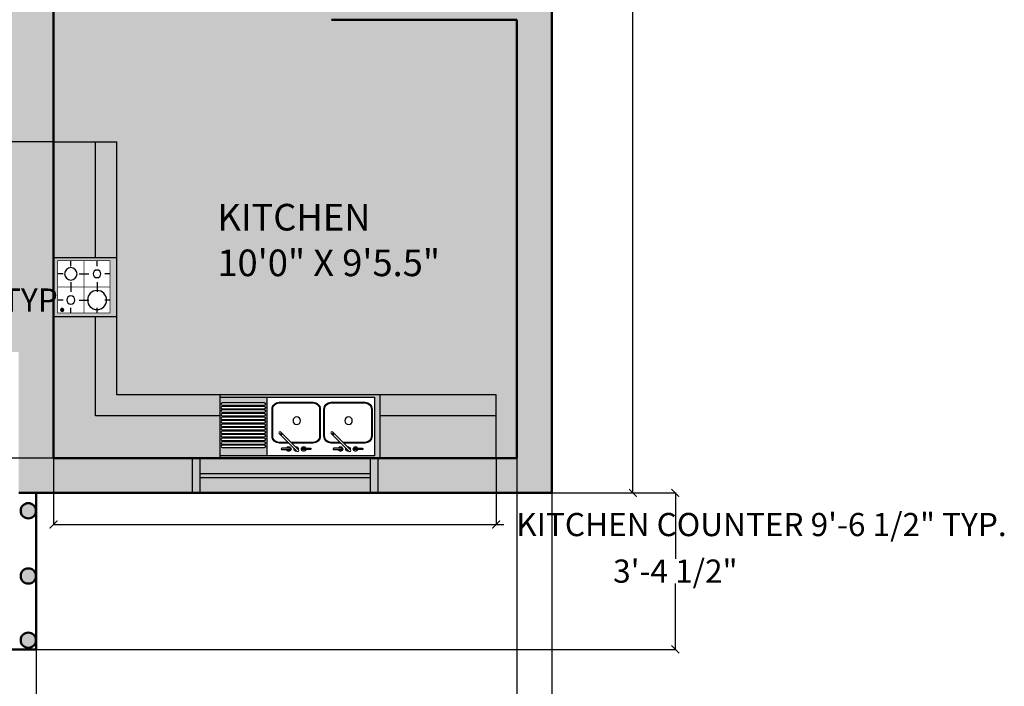
# Model space of a CAD drawing. Units: inches. Extents: x 528 to 2620, y -1066 to 798.
# Tile 23 of 41: x 1207 to 1462, y 219 to 391. Entities that reach past the tile are written whole.
import ezdxf

# ---------------------------------------------------------------- set-up
doc = ezdxf.new("R2010")
doc.units = ezdxf.units.IN
doc.header["$MEASUREMENT"] = 0
for name, color, linetype, lineweight in [('A-ANNO-DIMS', 2, 'Continuous', 18), ('A-AREA-IDEN', 7, 'Continuous', 18), ('A-FLOR-FIXT', 8, 'Continuous', 18), ('A-GLAZ', 3, 'Continuous', 25), ('A-WALL', 7, 'Continuous', 50), ('A-WALL-PATT', 8, 'Continuous', 13)]:
    doc.layers.add(name, color=color, linetype=linetype, lineweight=lineweight)
doc.layers.add('TEFRIS', color=11, linetype='Continuous')
doc.styles.get("Standard").update_dxf_attribs({"font": 'arial.ttf'})
doc.dimstyles.get("Standard").update_dxf_attribs({"dimtxt": 6, "dimasz": 2, "dimexe": 0.18, "dimexo": 0.0625, "dimgap": 0.09, "dimtad": 0, "dimtih": 1, "dimtoh": 1, "dimdec": 1, "dimzin": 0, "dimdsep": 46, "dimlunit": 3, "dimtxsty": 'Standard', "dimblk": 'ARCHTICK', "dimcen": 0.09, "dimadec": 0, "dimazin": 0, "dimtfac": 1, "dimtdec": 1, "dimtofl": 0, "dimtmove": 0, "dimatfit": 3, "dimfxl": 1, "dimtolj": 1, "dimtzin": 0, "dimarcsym": 0})

# ---------------------------------------------------------------- blocks, each defined once
blk = doc.blocks.new('A$C2CE61BFE')
at = {"layer": 'TEFRIS'}
for p, q in [((12.72, 49.97), (12.72, 44.98)), ((37.56, 49.97), (37.56, 44.98)), ((5.3, 37.56), (0.31, 37.56)), ((20.47, 37.56), (29.81, 37.56)), ((49.97, 37.56), (44.98, 37.56)), ((12.72, 20.47), (12.72, 29.81)), ((37.56, 20.47), (37.56, 29.81)), ((5.3, 12.72), (0.31, 12.72)), ((20.47, 12.72), (29.81, 12.72)), ((49.97, 12.72), (44.98, 12.72)), ((12.72, 5.3), (12.72, 0.31)), ((37.56, 5.3), (37.56, 0.31))]:
    blk.add_line(p, q, dxfattribs=at)
at = {"layer": 'TEFRIS', "const_width": 0.617}
blk.add_lwpolyline([(49.97, 49.97), (0.31, 49.97), (0.31, 0.31), (49.97, 0.31)], close=True, dxfattribs=at)
at = {"layer": 'TEFRIS', "const_width": 0.514}
for points in [[(25.14, 49.97), (25.14, 0.31)], [(49.97, 25.14), (0.31, 25.14)]]:
    blk.add_lwpolyline(points, dxfattribs=at)
at = {"layer": 'TEFRIS'}
for centre, radius in [((12.72, 37.56), 3.83), ((37.56, 37.56), 9.04), ((12.72, 12.72), 5.97), ((37.56, 12.72), 3.62)]:
    blk.add_circle(centre, radius, dxfattribs=at)
blk = doc.blocks.new('A$C59F64124')
at = {"layer": 'TEFRIS'}
for p, q in [((0, 0), (0, 60)), ((146.83, 57.74), (0, 57.74)), ((44.54, 2.06), (44.54, 57.74)), ((146.83, 2.06), (146.83, 57.74)), ((0, 2.06), (146.83, 2.06))]:
    blk.add_line(p, q, dxfattribs=at)
for points in [[(2.23, 49.95), (42.31, 49.95, -1), (42.31, 47.72), (2.23, 47.72, -1), (2.23, 49.95)], [(2.23, 46.61), (42.31, 46.61, -1), (42.31, 44.38), (2.23, 44.38, -1), (2.23, 46.61)], [(2.23, 43.27), (42.31, 43.27, -1), (42.31, 41.04), (2.23, 41.04, -1), (2.23, 43.27)], [(2.23, 39.92), (42.31, 39.92, -1), (42.31, 37.7), (2.23, 37.7, -1), (2.23, 39.92)], [(65.32, 45.72), (56.17, 45.72, 0.414214), (49.49, 39.04)], [(49.49, 39.04), (49.49, 13.7, 0.414214), (56.17, 7.01), (88.58, 7.01, 0.414214), (95.26, 13.7), (95.26, 39.04, 0.414214), (88.58, 45.72), (68.32, 45.72, 0.414214)], [(64.66, 45.05), (56.17, 45.05, 0.414214), (50.15, 39.04)], [(50.15, 39.04), (50.15, 13.7, 0.414214), (56.17, 7.68), (88.58, 7.68, 0.414214), (94.6, 13.7), (94.6, 39.04, 0.414214), (88.58, 45.05), (67.66, 45.05, 0.414214)], [(114.49, 45.72), (105.34, 45.72, 0.414214), (98.65, 39.04)], [(98.65, 39.04), (98.65, 13.7, 0.414214), (105.34, 7.01), (137.75, 7.01, 0.414214), (144.43, 13.7), (144.43, 39.04, 0.414214), (137.75, 45.72), (117.49, 45.72, 0.330435)], [(113.83, 45.05), (105.34, 45.05, 0.414214), (99.32, 39.04)], [(99.32, 39.04), (99.32, 13.7, 0.414214), (105.34, 7.68), (137.75, 7.68, 0.414214), (143.77, 13.7), (143.77, 39.04, 0.414214), (137.75, 45.05), (116.83, 45.05, 0.333106)], [(2.23, 36.58), (42.31, 36.58, -1), (42.31, 34.36), (2.23, 34.36, -1), (2.23, 36.58)], [(2.23, 33.24), (42.31, 33.24, -1), (42.31, 31.02), (2.23, 31.02, -1), (2.23, 33.24)], [(2.23, 29.9), (42.31, 29.9, -1), (42.31, 27.68), (2.23, 27.68, -1), (2.23, 29.9)], [(2.23, 26.56), (42.31, 26.56, -1), (42.31, 24.34), (2.23, 24.34, -1), (2.23, 26.56)], [(2.23, 23.22), (42.31, 23.22, -1), (42.31, 20.99), (2.23, 20.99, -1), (2.23, 23.22)], [(2.23, 19.88), (42.31, 19.88, -1), (42.31, 17.65), (2.23, 17.65, -1), (2.23, 19.88)], [(2.23, 16.54), (42.31, 16.54, -1), (42.31, 14.31), (2.23, 14.31, -1), (2.23, 16.54)], [(2.23, 13.2), (42.31, 13.2, -1), (42.31, 10.97), (2.23, 10.97, -1), (2.23, 13.2)], [(2.23, 9.86), (42.31, 9.86, -1), (42.31, 7.63), (2.23, 7.63, -1), (2.23, 9.86)]]:
    blk.add_lwpolyline(points, format="xyb", dxfattribs=at)
for points in [[(56.35, 36.75), (73.1, 53.5, -1), (74.6, 52), (57.85, 35.25, -1)], [(58.87, 51.96), (66.5, 51.96, -0.563183), (66.5, 50.54), (58.87, 50.54, -1)], [(85.83, 51.96), (78.2, 51.96, 0.563183), (78.2, 50.54), (85.83, 50.54, 1)], [(105.52, 36.75), (122.27, 53.5, -1), (123.77, 52), (107.02, 35.25, -1)], [(108.04, 51.96), (115.67, 51.96, -0.563183), (115.67, 50.54), (108.04, 50.54, -1)], [(135, 51.96), (127.37, 51.96, 0.563183), (127.37, 50.54), (135, 50.54, 1)]]:
    blk.add_lwpolyline(points, format="xyb", close=True, dxfattribs=at)
for centre, radius in [((58.21, 37.11), 0.707), ((107.38, 37.11), 0.707), ((72.91, 24.51), 3.54), ((122.08, 24.51), 3.54)]:
    blk.add_circle(centre, radius, dxfattribs=at)
for centre, start, end in [((65.24, 51.25), 199.47122, 160.52878), ((72.35, 51.25), 75, 195), ((72.35, 51.25), 255, 15), ((79.47, 51.25), 19.47122, 340.52878), ((114.41, 51.25), 199.47122, 160.52878), ((121.52, 51.25), 75, 195), ((121.52, 51.25), 255, 15), ((128.64, 51.25), 19.47122, 340.52878)]:
    blk.add_arc(centre, 2.12, start, end, dxfattribs=at)
blk = doc.blocks.new('A$C344845E7')
at = {"layer": 'TEFRIS'}
for p, q in [((-0.6, 4.2), (-0.6, 0.6)), ((0, 4.2), (-0.6, 4.2)), ((-0.4, 4.2), (-0.4, 3.1)), ((0, 0), (0, 4.2)), ((0, 3.1), (-0.6, 3.1)), ((-0.4, 1.5788), (-0.4, 0.4)), ((-2.9993, 0), (-2.9993, 0.6)), ((-0.6, 0.6), (-2.9993, 0.6)), ((-1.9, 0.6), (-1.9, 0)), ((-1.3397, 0.6), (-1.3397, 0)), ((-1.9, 0.4), (-2.9993, 0.4)), ((-0.4, 0.4), (-1.3397, 0.4)), ((0, 0), (-2.9993, 0))]:
    blk.add_line(p, q, dxfattribs=at)
at = {"layer": 'TEFRIS', "xscale": -0.01, "yscale": 0.01, "zscale": 0.01, "rotation": 270}
for name, p in [('A$C59F64124', (-0.6, 1.5788)), ('A$C2CE61BFE', (-1.8756, 0.0373))]:
    blk.add_blockref(name, p, dxfattribs=at)
blk = doc.blocks.new('_ArchTick')
at = {"color": 0, "linetype": 'ByBlock', "const_width": 0.15}
blk.add_lwpolyline([(-0.5, -0.5), (0.5, 0.5)], dxfattribs=at)
blk = doc.blocks.new('*D17')
at = {"layer": 'A-ANNO-DIMS', "color": 0, "lineweight": -2, "transparency": 16777216}
for p, q in [((1345.06, 718.92), (1366.18, 718.92)), ((1366, 718.92), (1366, 497.08)), ((1366, 268.92), (1366, 490.77)), ((1345.06, 268.92), (1366.18, 268.92))]:
    blk.add_line(p, q, dxfattribs=at)
at = {"layer": 'Defpoints', "color": 0, "transparency": 16777216}
for p in [(1345, 718.92), (1345, 268.92), (1366, 268.92)]:
    blk.add_point(p, dxfattribs=at)
at = {"layer": 'A-ANNO-DIMS', "color": 0, "lineweight": -2, "transparency": 16777216, "xscale": 2, "yscale": 2, "zscale": 2}
for p, rotation in [((1366, 718.92), 90), ((1366, 268.92), 270)]:
    blk.add_blockref('_ArchTick', p, dxfattribs=dict(at, rotation=rotation))
at = {"layer": 'A-ANNO-DIMS', "color": 0, "transparency": 16777216, "insert": (1366, 493.92), "char_height": 6, "attachment_point": 5}
blk.add_mtext('\\A1;37\'-6.0"', dxfattribs=at)
blk = doc.blocks.new('WIN-1200')
for p, q in [((677.56, 718.92), (725.56, 718.92)), ((677.56, 709.92), (677.56, 718.92)), ((679.56, 709.92), (679.56, 718.92)), ((723.56, 718.92), (723.56, 709.92)), ((725.56, 718.92), (725.56, 709.92)), ((679.56, 714.92), (723.56, 714.92)), ((679.56, 713.92), (723.56, 713.92)), ((725.56, 709.92), (677.56, 709.92))]:
    blk.add_line(p, q)
blk = doc.blocks.new('*D46')
at = {"layer": 'A-ANNO-DIMS', "color": 0, "lineweight": -2, "transparency": 16777216}
for p, q in [((1216, 277.86), (1216, 260.55)), ((1330.61, 277.86), (1330.61, 260.55)), ((1216, 260.73), (1330.61, 260.73)), ((1330.61, 260.73), (1332.61, 260.73))]:
    blk.add_line(p, q, dxfattribs=at)
at = {"layer": 'Defpoints', "color": 0, "transparency": 16777216}
for p in [(1216, 277.92), (1330.61, 277.92), (1330.61, 260.73)]:
    blk.add_point(p, dxfattribs=at)
at = {"layer": 'A-ANNO-DIMS', "color": 0, "lineweight": -2, "transparency": 16777216, "xscale": 2, "yscale": 2, "zscale": 2, "rotation": 180}
blk.add_blockref('_ArchTick', (1216, 260.73), dxfattribs=at)
at = {"layer": 'A-ANNO-DIMS', "color": 0, "lineweight": -2, "transparency": 16777216, "xscale": 2, "yscale": 2, "zscale": 2}
blk.add_blockref('_ArchTick', (1330.61, 260.73), dxfattribs=at)
at = {"layer": 'A-ANNO-DIMS', "color": 0, "transparency": 16777216, "insert": (1399.29, 260.73), "char_height": 6, "attachment_point": 5}
blk.add_mtext('\\A1;KITCHEN COUNTER 9\'-6 1/2" TYP.', dxfattribs=at)
blk = doc.blocks.new('*D47')
at = {"layer": 'A-ANNO-DIMS', "color": 0, "lineweight": -2, "transparency": 16777216}
for p, q in [((1215.93, 359.77), (1198.62, 359.77)), ((1198.8, 359.77), (1198.8, 322)), ((1198.8, 277.92), (1198.8, 315.69)), ((1215.93, 277.92), (1198.62, 277.92))]:
    blk.add_line(p, q, dxfattribs=at)
at = {"layer": 'Defpoints', "color": 0, "transparency": 16777216}
for p in [(1216, 359.77), (1198.8, 277.92), (1216, 277.92)]:
    blk.add_point(p, dxfattribs=at)
at = {"layer": 'A-ANNO-DIMS', "color": 0, "lineweight": -2, "transparency": 16777216, "xscale": 2, "yscale": 2, "zscale": 2}
for p, rotation in [((1198.8, 359.77), 90), ((1198.8, 277.92), 270)]:
    blk.add_blockref('_ArchTick', p, dxfattribs=dict(at, rotation=rotation))
at = {"layer": 'A-ANNO-DIMS', "color": 0, "transparency": 16777216, "insert": (1198.8, 318.84), "char_height": 6, "attachment_point": 5}
blk.add_mtext('\\A1;6\'-10" TYP.', dxfattribs=at)
blk = doc.blocks.new('*D60')
at = {"layer": 'A-ANNO-DIMS', "color": 0, "lineweight": -2, "transparency": 16777216}
for p, q in [((1024.5, 228.36), (1024.5, 196.24)), ((1211.5, 228.36), (1211.5, 196.24)), ((1024.5, 196.42), (1107.88, 196.42)), ((1211.5, 196.42), (1128.11, 196.42))]:
    blk.add_line(p, q, dxfattribs=at)
at = {"layer": 'Defpoints', "color": 0, "transparency": 16777216}
for p in [(1024.5, 228.42), (1211.5, 228.42), (1211.5, 196.42)]:
    blk.add_point(p, dxfattribs=at)
at = {"layer": 'A-ANNO-DIMS', "color": 0, "lineweight": -2, "transparency": 16777216, "xscale": 2, "yscale": 2, "zscale": 2, "rotation": 180}
blk.add_blockref('_ArchTick', (1024.5, 196.42), dxfattribs=at)
at = {"layer": 'A-ANNO-DIMS', "color": 0, "lineweight": -2, "transparency": 16777216, "xscale": 2, "yscale": 2, "zscale": 2}
blk.add_blockref('_ArchTick', (1211.5, 196.42), dxfattribs=at)
at = {"layer": 'A-ANNO-DIMS', "color": 0, "transparency": 16777216, "insert": (1118, 196.42), "char_height": 6, "attachment_point": 5}
blk.add_mtext('\\A1;15\'-7"', dxfattribs=at)
blk = doc.blocks.new('*D61')
at = {"layer": 'A-ANNO-DIMS', "color": 0, "lineweight": -2, "transparency": 16777216}
for p, q in [((1336, 277.86), (1336, 196.24)), ((1211.5, 228.36), (1211.5, 196.24)), ((1211.5, 196.42), (1256.64, 196.42)), ((1336, 196.42), (1290.85, 196.42))]:
    blk.add_line(p, q, dxfattribs=at)
at = {"layer": 'Defpoints', "color": 0, "transparency": 16777216}
for p in [(1336, 277.92), (1211.5, 228.42), (1336, 196.42)]:
    blk.add_point(p, dxfattribs=at)
at = {"layer": 'A-ANNO-DIMS', "color": 0, "lineweight": -2, "transparency": 16777216, "xscale": 2, "yscale": 2, "zscale": 2, "rotation": 180}
blk.add_blockref('_ArchTick', (1211.5, 196.42), dxfattribs=at)
at = {"layer": 'A-ANNO-DIMS', "color": 0, "lineweight": -2, "transparency": 16777216, "xscale": 2, "yscale": 2, "zscale": 2}
blk.add_blockref('_ArchTick', (1336, 196.42), dxfattribs=at)
at = {"layer": 'A-ANNO-DIMS', "color": 0, "transparency": 16777216, "insert": (1273.75, 196.42), "char_height": 6, "attachment_point": 5}
blk.add_mtext('\\A1;10\'-4 1/2"', dxfattribs=at)
blk = doc.blocks.new('*D62')
at = {"layer": 'A-ANNO-DIMS', "color": 0, "lineweight": -2, "transparency": 16777216}
for p, q in [((1336, 277.86), (1336, 196.24)), ((1345, 268.86), (1345, 196.24)), ((1336, 196.42), (1345, 196.42)), ((1345, 196.42), (1347, 196.42))]:
    blk.add_line(p, q, dxfattribs=at)
at = {"layer": 'Defpoints', "color": 0, "transparency": 16777216}
for p in [(1336, 277.92), (1345, 268.92), (1345, 196.42)]:
    blk.add_point(p, dxfattribs=at)
at = {"layer": 'A-ANNO-DIMS', "color": 0, "lineweight": -2, "transparency": 16777216, "xscale": 2, "yscale": 2, "zscale": 2, "rotation": 180}
blk.add_blockref('_ArchTick', (1336, 196.42), dxfattribs=at)
at = {"layer": 'A-ANNO-DIMS', "color": 0, "lineweight": -2, "transparency": 16777216, "xscale": 2, "yscale": 2, "zscale": 2}
blk.add_blockref('_ArchTick', (1345, 196.42), dxfattribs=at)
at = {"layer": 'A-ANNO-DIMS', "color": 0, "transparency": 16777216, "insert": (1355.06, 196.42), "char_height": 6, "attachment_point": 5}
blk.add_mtext('\\A1;0\'-9"', dxfattribs=at)
blk = doc.blocks.new('*D65')
at = {"layer": 'A-ANNO-DIMS', "color": 0, "lineweight": -2, "transparency": 16777216}
for p, q in [((1211.56, 268.92), (1377.18, 268.92)), ((1377, 268.92), (1377, 251.87)), ((1377, 228.42), (1377, 245.48)), ((1211.56, 228.42), (1377.18, 228.42))]:
    blk.add_line(p, q, dxfattribs=at)
at = {"layer": 'Defpoints', "color": 0, "transparency": 16777216}
for p in [(1211.5, 268.92), (1211.5, 228.42), (1377, 228.42)]:
    blk.add_point(p, dxfattribs=at)
at = {"layer": 'A-ANNO-DIMS', "color": 0, "lineweight": -2, "transparency": 16777216, "xscale": 2, "yscale": 2, "zscale": 2}
for p, rotation in [((1377, 268.92), 90), ((1377, 228.42), 270)]:
    blk.add_blockref('_ArchTick', p, dxfattribs=dict(at, rotation=rotation))
at = {"layer": 'A-ANNO-DIMS', "color": 0, "transparency": 16777216, "insert": (1377, 248.67), "char_height": 6, "attachment_point": 5}
blk.add_mtext('\\A1;3\'-4 1/2"', dxfattribs=at)

msp = doc.modelspace()

# ---------------------------------------------------------------- hatches: boundary and pattern name
at = {"layer": 'A-WALL-PATT', "transparency": 33554521}
h = msp.add_hatch(color=256, dxfattribs=at)
h.dxf.hatch_style = 1
h.paths.add_polyline_path([(1066, 709.92), (1114.5, 709.92), (1114.5, 718.92), (1057, 718.92), (1057, 667.92), (1066, 667.92)])
h.paths.add_polyline_path([(1227.5, 718.92), (1162.5, 718.92), (1162.5, 709.92), (1211, 709.92), (1211, 577.92), (1205.42, 577.92), (1205.5, 573.42), (1211, 573.42), (1211, 567.42), (1215.5, 567.42), (1215.5, 669.42), (1268, 669.42), (1268, 675.92), (1263.5, 675.92), (1263.5, 673.92), (1215.5, 673.92), (1215.5, 709.92), (1227.5, 709.92)])
h.paths.add_polyline_path([(1345, 718.92), (1316, 718.92), (1316, 709.92), (1336, 709.92), (1336, 641.67), (1345, 641.67)])
h.paths.add_polyline_path([(1066, 619.92), (1057, 619.92), (1057, 561.42), (1066, 561.42), (1066, 573.42), (1161, 573.42), (1161, 569.42), (1165.5, 569.42), (1165.5, 577.92), (1066, 577.92)])
h.paths.add_polyline_path([(1216, 391.42), (1216, 400.42), (1207, 400.42), (1201, 400.42), (1201, 397.42), (1201, 391.42), (1207, 391.42), (1207, 268.92), (1252, 268.92), (1252, 277.92), (1216, 277.92), (1216, 359.77)])
h.paths.add_polyline_path([(1345, 395.92), (1336, 395.92), (1288, 395.92), (1288, 391.42), (1336, 391.42), (1336, 277.92), (1300, 277.92), (1300, 268.92), (1345, 268.92)])
h.paths.add_polyline_path([(1345, 593.67), (1336, 593.67), (1336, 525.42), (1215.5, 525.42), (1215.5, 527.17), (1211, 527.17), (1211, 520.92), (1336, 520.92), (1336, 443.92), (1345, 443.92)])
h.paths.add_polyline_path([(1066, 520.92), (1165.5, 520.92), (1165.5, 545.42), (1161, 545.42), (1161, 525.42), (1066, 525.42), (1066, 537.42), (1057, 537.42), (1057, 484.67), (1066, 484.67)])
h.paths.add_polyline_path([(1066, 436.67), (1057, 436.67), (1057, 391.42), (1085.5, 391.42), (1085.5, 400.42), (1066, 400.42)])
h.paths.add_polyline_path([(1153, 397.42), (1153, 400.42), (1133.5, 400.42), (1133.5, 391.42), (1153, 391.42)])
at = {"layer": 'A-WALL-PATT', "transparency": 33554681}
h = msp.add_hatch(color=256, dxfattribs=at)
h.dxf.hatch_style = 1
h.paths.add_polyline_path([(1066, 665.92), (1062, 665.92), (1062, 621.92), (1066, 621.92)])
h.paths.add_polyline_path([(1061, 665.92), (1057, 665.92), (1057, 621.92), (1061, 621.92)])
h.paths.add_polyline_path([(1160.5, 713.92), (1116.5, 713.92), (1116.5, 709.92), (1160.5, 709.92)])
h.paths.add_polyline_path([(1160.5, 718.92), (1116.5, 718.92), (1116.5, 714.92), (1160.5, 714.92)])
h.paths.add_polyline_path([(1251.5, 713.92), (1227.5, 713.92), (1227.5, 709.92), (1251.5, 709.92)])
h.paths.add_polyline_path([(1251.5, 718.92), (1227.5, 718.92), (1227.5, 714.92), (1251.5, 714.92)])
h.paths.add_polyline_path([(1314, 713.92), (1270, 713.92), (1270, 709.92), (1314, 709.92)])
h.paths.add_polyline_path([(1314, 718.92), (1270, 718.92), (1270, 714.92), (1314, 714.92)])
h.paths.add_polyline_path([(1345, 639.67), (1341, 639.67), (1341, 595.67), (1345, 595.67)])
h.paths.add_polyline_path([(1340, 639.67), (1336, 639.67), (1336, 595.67), (1340, 595.67)])
h.paths.add_polyline_path([(1345, 441.92), (1341, 441.92), (1341, 397.92), (1345, 397.92)])
h.paths.add_polyline_path([(1340, 441.92), (1336, 441.92), (1336, 397.92), (1340, 397.92)])
h.paths.add_polyline_path([(1298, 272.92), (1254, 272.92), (1254, 268.92), (1298, 268.92)])
h.paths.add_polyline_path([(1298, 277.92), (1254, 277.92), (1254, 273.92), (1298, 273.92)])
h.paths.add_polyline_path([(1131.5, 395.42), (1087.5, 395.42), (1087.5, 391.42), (1131.5, 391.42)])
h.paths.add_polyline_path([(1131.5, 400.42), (1087.5, 400.42), (1087.5, 396.42), (1131.5, 396.42)])
h.paths.add_polyline_path([(1066, 482.67), (1062, 482.67), (1062, 438.67), (1066, 438.67)])
h.paths.add_polyline_path([(1061, 482.67), (1057, 482.67), (1057, 438.67), (1061, 438.67)])
h.paths.add_polyline_path([(1066, 561.42), (1062, 561.42), (1062, 537.42), (1066, 537.42)])
h.paths.add_polyline_path([(1061, 561.42), (1057, 561.42), (1057, 537.42), (1061, 537.42)])
at = {"layer": 'A-WALL-PATT', "transparency": 33554536}
h = msp.add_hatch(color=256, dxfattribs=at)
h.dxf.hatch_style = 1
h.paths.add_polyline_path([(1336, 709.92), (1268, 709.92), (1268, 699.92), (1266.75, 699.92), (1266.75, 675.92), (1268, 675.92), (1268, 669.42), (1215.5, 669.42), (1215.5, 567.17), (1217, 567.17), (1257, 567.17), (1257, 565.42), (1256.96, 565.42, -0.401453), (1217, 527.17), (1215.5, 527.17), (1215.5, 525.42), (1336, 525.42)], flags=17)
h.paths.add_polyline_path([(1285.03, 635.93), (1285.23, 636.13), (1285.67, 636.26), (1286.21, 636.02), (1286.98, 636.08), (1332.98, 636.08), (1333.36, 636.22), (1333.82, 636.08), (1334.11, 635.71), (1334.11, 635.3), (1333.91, 634.86), (1333.82, 634.83), (1333.82, 592.74), (1333.97, 592.6), (1334.11, 592.29), (1334.11, 591.88), (1333.82, 591.51), (1333.36, 591.37), (1332.98, 591.51), (1332.64, 591.79), (1332.64, 591.51), (1286.98, 591.51), (1286.17, 591.67), (1286.07, 591.57), (1285.68, 591.37), (1285.23, 591.51), (1285.03, 591.71), (1284.83, 592.1), (1284.98, 592.54), (1285.13, 592.69), (1285.13, 634.95), (1284.98, 635.1), (1284.83, 635.54)], flags=16)
h.paths.add_polyline_path([(1285.03, 635.93), (1285.23, 636.13), (1285.67, 636.26), (1286.21, 636.02), (1286.98, 636.08), (1332.98, 636.08), (1333.36, 636.22), (1333.82, 636.08), (1334.11, 635.71), (1334.11, 635.3), (1333.97, 634.99), (1333.82, 634.85), (1333.82, 592.74), (1333.97, 592.6), (1334.11, 592.29), (1334.11, 591.88), (1333.82, 591.51), (1333.36, 591.37), (1332.98, 591.51), (1332.64, 591.79), (1332.64, 592.25), (1332.64, 635.35), (1332.64, 635.8), (1332.98, 636.08), (1312.23, 636.08), (1311.1, 635.48), (1310.63, 635.48), (1310.43, 635.23), (1309.94, 635.1), (1309.7, 634.99), (1309.06, 634.76), (1308.71, 634.61), (1308.32, 634.61), (1307.75, 634.36), (1307.11, 634.27), (1307.01, 634.11), (1306.77, 634.02), (1307.25, 633.28), (1306.87, 633.04), (1306.77, 632.88), (1306.37, 632.64), (1306.03, 632.55), (1305.54, 632.41), (1315.47, 618.49), (1316.32, 619.39), (1312.77, 622.86), (1319.62, 630.11), (1320.07, 629.68), (1320.11, 630), (1320.28, 630.6), (1320.53, 631.18), (1320.53, 632.01), (1320.26, 632.55), (1320.11, 633.13), (1320.06, 633.73), (1320.63, 634.02), (1321.22, 634.16), (1321.86, 634.11), (1322.45, 633.91), (1322.99, 633.62), (1324.1, 633.62), (1324.64, 633.91), (1325.23, 634.07), (1325.87, 634.07), (1326.43, 633.91), (1326.98, 633.62), (1328.35, 633.62), (1328.9, 633.91), (1329.49, 634.11), (1330.1, 634.16), (1330.69, 634.02), (1331.28, 633.73), (1331.23, 633.13), (1331.09, 632.55), (1330.79, 632.01), (1330.79, 631.18), (1331.04, 630.6), (1331.23, 630), (1331.28, 629.41), (1331.19, 628.79), (1331.04, 628.18), (1330.79, 627.6), (1330.79, 626.77), (1331.04, 626.19), (1331.23, 625.59), (1331.28, 625.01), (1331.19, 624.38), (1331.04, 623.78), (1330.79, 623.24), (1330.79, 622.37), (1331.04, 621.83), (1331.23, 621.25), (1331.28, 620.6), (1331.19, 619.97), (1331.04, 619.37), (1330.79, 618.83), (1330.79, 617.96), (1331.09, 617.42), (1331.23, 616.88), (1331.28, 616.23), (1331.28, 615.52), (1330.69, 615.27), (1330.1, 615.12), (1329.49, 615.12), (1328.9, 615.32), (1328.35, 615.65), (1326.98, 615.65), (1326.43, 615.32), (1325.87, 615.16), (1325.23, 615.16), (1324.64, 615.32), (1324.1, 615.65), (1323.24, 615.65), (1324.93, 614.04), (1322.98, 611.98), (1324.1, 611.98), (1324.64, 612.27), (1325.28, 612.43), (1325.87, 612.43), (1326.48, 612.27), (1327.03, 611.98), (1328.35, 611.98), (1328.9, 612.27), (1329.49, 612.48), (1330.1, 612.52), (1330.74, 612.39), (1331.28, 612.07), (1331.28, 611.36), (1331.28, 610.75), (1331.09, 610.17), (1330.79, 609.63), (1330.79, 608.81), (1331.09, 608.22), (1331.23, 607.62), (1331.28, 606.99), (1331.23, 606.41), (1331.09, 605.81), (1330.79, 605.22), (1330.79, 604.4), (1331.09, 603.81), (1331.23, 603.21), (1331.28, 602.63), (1331.23, 602), (1331.09, 601.4), (1330.79, 600.86), (1330.79, 599.99), (1331.09, 599.45), (1331.23, 598.87), (1331.28, 598.22), (1331.23, 597.59), (1331.09, 596.99), (1330.79, 596.45), (1330.79, 595.58), (1331.09, 595.04), (1331.28, 594.51), (1331.28, 593.86), (1330.74, 593.61), (1330.1, 593.48), (1329.49, 593.48), (1328.9, 593.68), (1328.35, 594.01), (1327.03, 594.01), (1326.48, 593.68), (1325.87, 593.52), (1325.28, 593.52), (1324.64, 593.68), (1324.1, 594.01), (1323.04, 594.01), (1322.5, 593.68), (1321.91, 593.48), (1321.27, 593.48), (1320.63, 593.61), (1320.11, 593.86), (1320.11, 594.51), (1320.28, 595.04), (1320.58, 595.58), (1320.58, 596.45), (1320.28, 596.99), (1320.16, 597.59), (1320.1, 598.01), (1319.62, 597.55), (1315.66, 601.73), (1312.23, 591.57), (1311.74, 591.66), (1311.59, 591.91), (1310.78, 592.4), (1309.55, 592.89), (1308.96, 592.89), (1308.71, 593.03), (1308.56, 593.14), (1307.75, 593.52), (1306.77, 593.61), (1307.25, 594.36), (1306.87, 594.6), (1306.37, 594.84), (1306.03, 595.09), (1305.54, 595.24), (1315.46, 609.35), (1310.93, 613.71), (1315.47, 618.49), (1305.54, 632.41), (1306.03, 632.55), (1306.37, 632.64), (1306.77, 632.88), (1306.87, 633.04), (1307.25, 633.28), (1306.77, 634.02), (1307.01, 634.11), (1307.11, 634.27), (1307.75, 634.36), (1308.32, 634.61), (1308.71, 634.61), (1309.06, 634.76), (1309.7, 634.99), (1309.94, 635.1), (1310.43, 635.23), (1310.63, 635.48), (1311.1, 635.48), (1312.23, 636.08), (1286.98, 636.08), (1286.22, 636.02), (1286.41, 635.44), (1286.21, 635.05), (1286.02, 634.85), (1285.87, 634.81), (1285.87, 592.84), (1286.15, 592.73), (1286.41, 592.19), (1286.23, 591.66), (1286.17, 591.67), (1286.07, 591.57), (1285.68, 591.37), (1285.23, 591.51), (1285.03, 591.71), (1284.83, 592.1), (1284.98, 592.54), (1285.13, 592.69), (1285.13, 634.95), (1284.98, 635.1), (1284.83, 635.54)], flags=0)
h.paths.add_polyline_path([(1322.5, 653.6), (1333.65, 653.6), (1333.65, 637.99), (1322.5, 637.99)], flags=16)
h.paths.add_polyline_path([(1323.62, 652.48), (1332.53, 652.48), (1332.53, 639.11), (1323.62, 639.11)], flags=0)
edge = h.paths.add_edge_path(flags=0)
edge.add_ellipse((1328.07, 645.79), major_axis=(2.24, 2.24), ratio=1, start_angle=405, end_angle=495, ccw=False)
edge.add_ellipse((1328.07, 645.79), major_axis=(2.24, 2.24), ratio=1, start_angle=675, end_angle=765, ccw=False)
edge.add_ellipse((1328.07, 645.79), major_axis=(2.24, 2.24), ratio=1, start_angle=585, end_angle=675, ccw=False)
edge.add_ellipse((1328.07, 645.79), major_axis=(2.24, 2.24), ratio=1, start_angle=495, end_angle=585, ccw=False)
h.paths.add_polyline_path([(1320.58, 628.39), (1320.33, 628.01), (1320.61, 628.55)], flags=0)
h.paths.add_polyline_path([(1317.89, 604.89), (1318.78, 604.64), (1319.76, 604.28), (1318.88, 604.53)], flags=0)
h.paths.add_polyline_path([(1320.33, 599.65), (1320.58, 599.25), (1320.58, 599.16)], flags=0)
h.paths.add_polyline_path([(1322.5, 589.6), (1333.65, 589.6), (1333.65, 573.99), (1322.5, 573.99)], flags=16)
h.paths.add_polyline_path([(1323.62, 588.48), (1332.53, 588.48), (1332.53, 575.11), (1323.62, 575.11)], flags=0)
edge = h.paths.add_edge_path(flags=0)
edge.add_ellipse((1328.07, 581.8), major_axis=(-2.24, 2.24), ratio=1, start_angle=-45, end_angle=45, ccw=False)
edge.add_ellipse((1328.07, 581.8), major_axis=(-2.24, 2.24), ratio=1, start_angle=-135, end_angle=-45, ccw=False)
edge.add_ellipse((1328.07, 581.8), major_axis=(-2.24, 2.24), ratio=1, start_angle=135, end_angle=-135, ccw=False)
edge.add_ellipse((1328.07, 581.8), major_axis=(-2.24, 2.24), ratio=1, start_angle=45, end_angle=135, ccw=False)
h.paths.add_polyline_path([(1264.75, 699.92), (1263.5, 699.92), (1263.5, 709.92), (1215.5, 709.92), (1215.5, 673.92), (1263.5, 673.92), (1263.5, 675.92), (1264.75, 675.92)], flags=16)
h.paths.add_polyline_path([(1162.19, 569.42), (1161, 569.42), (1161, 573.42), (1066, 573.42), (1066, 525.42), (1161, 525.42), (1161, 545.42), (1162.19, 545.42)])
h.paths.add_polyline_path([(1256.96, 565.42), (1257, 565.42), (1257, 567.17), (1217, 567.17), (1215.5, 567.17), (1215.5, 567.42), (1211, 567.42), (1211, 573.42), (1205.5, 573.42), (1205.42, 577.92), (1211, 577.92), (1211, 709.92), (1066, 709.92), (1066, 577.92), (1165.5, 577.92), (1165.5, 569.42), (1164.19, 569.42), (1164.19, 545.42), (1165.5, 545.42), (1165.5, 520.92), (1153, 520.92), (1153, 484.92), (1102, 484.92), (1102, 436.42), (1153, 436.42), (1153, 400.42), (1153, 391.42), (1201, 391.42), (1201, 400.42), (1207, 400.42), (1216, 400.42), (1216, 391.42), (1216, 277.92), (1336, 277.92), (1336, 391.42), (1288, 391.42), (1288, 395.92), (1336, 395.92), (1336, 443.92), (1336, 520.92), (1211, 520.92), (1211, 527.17), (1215.5, 527.17), (1217, 527.17, 0.401453)])
h.paths.add_polyline_path([(1167.25, 579.42), (1165.5, 579.42), (1165.5, 619.42), (1167.25, 619.42)], flags=16)
h.paths.add_polyline_path([(1227.97, 501.56), (1236.36, 502.03), (1236.36, 492.55), (1227.97, 493.02, -0.254069)], flags=16)
h.paths.add_polyline_path([(1243.34, 515.69, -0.254069), (1251.88, 515.69), (1252.35, 507.3), (1242.87, 507.3)], flags=16)
h.paths.add_polyline_path([(1239.18, 504.68), (1256.03, 504.68), (1256.03, 479.42), (1239.18, 479.42)], flags=16)
h.paths.add_polyline_path([(1227.97, 489.6), (1236.36, 490.07), (1236.36, 480.59), (1227.97, 481.06, -0.254069)], flags=16)
h.paths.add_polyline_path([(1197.2, 624.04), (1197.2, 639.64), (1208.35, 639.64), (1208.35, 624.04)], flags=16)
h.paths.add_polyline_path([(1198.32, 625.15), (1198.32, 638.53), (1207.23, 638.53), (1207.23, 625.15)], flags=0)
h.paths.add_polyline_path([(1258.85, 502.03), (1267.25, 501.56, -0.254069), (1267.25, 493.02), (1258.85, 492.55)], flags=16)
h.paths.add_polyline_path([(1271.59, 519.66), (1333.67, 519.66), (1333.67, 451.59), (1319.09, 451.59), (1319.09, 505.07), (1288.09, 505.07), (1284.45, 505.07, -0.883215), (1270.68, 514.19), (1270.68, 518.75, -0.414214)], flags=16)
h.paths.add_polyline_path([(1331.85, 517.83), (1331.85, 453.42), (1328.2, 453.42), (1328.2, 505.07), (1298.42, 505.07), (1298.42, 514.19), (1288.09, 514.19), (1288.09, 517.83)], flags=0)
h.paths.add_polyline_path([(1242.87, 476.8), (1252.35, 476.8), (1251.88, 468.41, -0.254069), (1243.34, 468.41)], flags=16)
h.paths.add_polyline_path([(1258.85, 490.07), (1267.25, 489.6, -0.254069), (1267.25, 481.06), (1258.85, 480.59)], flags=16)
h.paths.add_polyline_path([(1161.68, 641.55), (1160.87, 641.72), (1160.77, 641.62), (1160.38, 641.41), (1159.93, 641.55), (1159.73, 641.75), (1159.53, 642.14), (1159.68, 642.58), (1159.83, 642.73), (1159.83, 684.99), (1159.68, 685.14), (1159.53, 685.58), (1159.73, 685.97), (1159.93, 686.17), (1160.37, 686.31), (1160.91, 686.06), (1161.68, 686.13), (1207.68, 686.13), (1208.06, 686.27), (1208.52, 686.13), (1208.81, 685.76), (1208.81, 685.34), (1208.61, 684.9), (1208.52, 684.87), (1208.52, 642.78), (1208.67, 642.65), (1208.88, 642.2), (1208.72, 641.8), (1208.52, 641.55), (1208.06, 641.41), (1207.68, 641.55), (1207.34, 641.83), (1207.34, 641.55)], flags=16)
h.paths.add_polyline_path([(1186.93, 641.62), (1186.44, 641.71), (1186.29, 641.95), (1185.48, 642.45), (1184.25, 642.94), (1183.66, 642.94), (1183.41, 643.07), (1183.26, 643.18), (1182.45, 643.57), (1181.47, 643.65), (1181.95, 644.4), (1181.57, 644.64), (1181.07, 644.89), (1180.73, 645.13), (1180.24, 645.29), (1190.16, 659.4), (1185.63, 663.75), (1190.17, 668.54), (1180.24, 682.46), (1180.73, 682.59), (1181.07, 682.68), (1181.47, 682.93), (1181.57, 683.08), (1181.95, 683.33), (1181.47, 684.07), (1181.71, 684.16), (1181.81, 684.31), (1182.45, 684.4), (1183.02, 684.65), (1183.41, 684.65), (1183.76, 684.81), (1184.4, 685.03), (1184.64, 685.14), (1185.13, 685.28), (1185.33, 685.52), (1185.8, 685.52), (1186.93, 686.13), (1161.68, 686.13), (1160.92, 686.06), (1161.11, 685.49), (1160.91, 685.1), (1160.72, 684.9), (1160.57, 684.85), (1160.57, 642.88), (1160.85, 642.77), (1161.11, 642.23), (1160.93, 641.7), (1160.87, 641.72), (1160.77, 641.62), (1160.38, 641.41), (1159.93, 641.55), (1159.73, 641.75), (1159.53, 642.14), (1159.68, 642.58), (1159.83, 642.73), (1159.83, 684.99), (1159.68, 685.14), (1159.53, 685.58), (1159.73, 685.97), (1159.93, 686.17), (1160.37, 686.31), (1160.91, 686.06), (1161.68, 686.13), (1207.68, 686.13), (1208.06, 686.27), (1208.52, 686.13), (1208.81, 685.76), (1208.81, 685.34), (1208.67, 685.03), (1208.52, 684.9), (1208.52, 642.78), (1208.67, 642.65), (1208.88, 642.2), (1208.72, 641.8), (1208.52, 641.55), (1208.06, 641.41), (1207.68, 641.55), (1207.34, 641.83), (1207.34, 642.29), (1207.34, 685.39), (1207.34, 685.85), (1207.68, 686.13), (1186.93, 686.13), (1185.8, 685.52), (1185.33, 685.52), (1185.13, 685.28), (1184.64, 685.14), (1184.4, 685.03), (1183.76, 684.81), (1183.41, 684.65), (1183.02, 684.65), (1182.45, 684.4), (1181.81, 684.31), (1181.71, 684.16), (1181.47, 684.07), (1181.95, 683.33), (1181.57, 683.08), (1181.47, 682.93), (1181.07, 682.68), (1180.73, 682.59), (1180.24, 682.46), (1190.17, 668.54), (1191.02, 669.43), (1187.47, 672.9), (1194.32, 680.15), (1194.77, 679.72), (1194.81, 680.04), (1194.98, 680.65), (1195.23, 681.23), (1195.23, 682.05), (1194.96, 682.59), (1194.81, 683.17), (1194.76, 683.78), (1195.33, 684.07), (1195.92, 684.2), (1196.56, 684.16), (1197.15, 683.96), (1197.69, 683.67), (1198.8, 683.67), (1199.34, 683.96), (1199.93, 684.11), (1200.57, 684.11), (1201.13, 683.96), (1201.68, 683.67), (1203.05, 683.67), (1203.6, 683.96), (1204.19, 684.16), (1204.8, 684.2), (1205.39, 684.07), (1205.98, 683.78), (1205.93, 683.17), (1205.79, 682.59), (1205.49, 682.05), (1205.49, 681.23), (1205.74, 680.65), (1205.93, 680.04), (1205.98, 679.46), (1205.89, 678.83), (1205.74, 678.23), (1205.49, 677.65), (1205.49, 676.82), (1205.74, 676.24), (1205.93, 675.63), (1205.98, 675.05), (1205.89, 674.42), (1205.74, 673.82), (1205.49, 673.28), (1205.49, 672.41), (1205.74, 671.87), (1205.93, 671.29), (1205.98, 670.64), (1205.89, 670.02), (1205.74, 669.41), (1205.49, 668.87), (1205.49, 668), (1205.79, 667.46), (1205.93, 666.93), (1205.98, 666.28), (1205.98, 665.56), (1205.39, 665.32), (1204.8, 665.16), (1204.19, 665.16), (1203.6, 665.36), (1203.05, 665.7), (1201.68, 665.7), (1201.13, 665.36), (1200.57, 665.2), (1199.93, 665.2), (1199.34, 665.36), (1198.8, 665.7), (1197.94, 665.7), (1199.63, 664.09), (1197.68, 662.03), (1198.8, 662.03), (1199.34, 662.32), (1199.98, 662.47), (1200.57, 662.47), (1201.18, 662.32), (1201.73, 662.03), (1203.05, 662.03), (1203.6, 662.32), (1204.19, 662.52), (1204.8, 662.56), (1205.44, 662.43), (1205.98, 662.12), (1205.98, 661.4), (1205.98, 660.8), (1205.79, 660.21), (1205.49, 659.68), (1205.49, 658.85), (1205.79, 658.27), (1205.93, 657.66), (1205.98, 657.04), (1205.93, 656.45), (1205.79, 655.85), (1205.49, 655.27), (1205.49, 654.44), (1205.79, 653.86), (1205.93, 653.25), (1205.98, 652.67), (1205.93, 652.05), (1205.79, 651.44), (1205.49, 650.91), (1205.49, 650.03), (1205.79, 649.5), (1205.93, 648.91), (1205.98, 648.26), (1205.93, 647.64), (1205.79, 647.03), (1205.49, 646.5), (1205.49, 645.62), (1205.79, 645.09), (1205.98, 644.55), (1205.98, 643.9), (1205.44, 643.65), (1204.8, 643.52), (1204.19, 643.52), (1203.6, 643.72), (1203.05, 644.06), (1201.73, 644.06), (1201.18, 643.72), (1200.57, 643.57), (1199.98, 643.57), (1199.34, 643.72), (1198.8, 644.06), (1197.74, 644.06), (1197.2, 643.72), (1196.61, 643.52), (1195.97, 643.52), (1195.33, 643.65), (1194.81, 643.9), (1194.81, 644.55), (1194.98, 645.09), (1195.28, 645.62), (1195.28, 646.5), (1194.98, 647.03), (1194.86, 647.64), (1194.8, 648.06), (1194.32, 647.59), (1190.36, 651.77)], flags=16)
h.paths.add_polyline_path([(1195.28, 649.2), (1195.03, 649.7), (1195.28, 649.29)], flags=0)
h.paths.add_polyline_path([(1194.46, 654.33), (1193.58, 654.58), (1192.59, 654.93), (1193.48, 654.69)], flags=0)
h.paths.add_polyline_path([(1195.28, 678.43), (1195.03, 678.05), (1195.31, 678.59)], flags=0)
h.paths.add_polyline_path([(1197.2, 688.04), (1197.2, 703.64), (1208.35, 703.64), (1208.35, 688.04)], flags=16)
h.paths.add_polyline_path([(1198.32, 689.15), (1198.32, 702.53), (1207.23, 702.53), (1207.23, 689.15)], flags=0)
h.paths.add_polyline_path([(1217.1, 329.02), (1230.65, 329.02), (1230.65, 315.47), (1217.1, 315.47)], flags=16)
h.paths.add_polyline_path([(1223.87, 322.24), (1227.26, 322.24), (1227.26, 321.32, -0.414214), (1229.73, 318.86, -1), (1224.8, 318.86), (1223.87, 318.86)], flags=0)
h.paths.add_polyline_path([(1222.11, 325.63, -1), (1218.86, 325.63, -1)], flags=0)
h.paths.add_polyline_path([(1228.25, 325.63, -1), (1226.28, 325.63, -1)], flags=0)
h.paths.add_polyline_path([(1221.53, 318.86, -1), (1219.44, 318.86, -1)], flags=0)
h.paths.add_polyline_path([(1299.15, 293.73), (1299.15, 278.54), (1271.23, 278.54), (1271.23, 293.73)], flags=16)
h.paths.add_polyline_path([(1259.69, 292.21), (1270.62, 292.21, -1), (1270.62, 291.6), (1259.69, 291.6, -1)], flags=16)
h.paths.add_polyline_path([(1259.69, 291.3), (1270.62, 291.3, -1), (1270.62, 290.69), (1259.69, 290.69, -1)], flags=16)
h.paths.add_polyline_path([(1259.69, 290.39), (1270.62, 290.39, -1), (1270.62, 289.78), (1259.69, 289.78, -1)], flags=16)
h.paths.add_polyline_path([(1259.69, 289.48), (1270.62, 289.48, -1), (1270.62, 288.87), (1259.69, 288.87, -1)], flags=16)
h.paths.add_polyline_path([(1259.69, 288.57), (1270.62, 288.57, -1), (1270.62, 287.96), (1259.69, 287.96, -1)], flags=16)
h.paths.add_polyline_path([(1274.41, 292.38), (1283.25, 292.38, -0.414214), (1285.07, 290.56), (1285.07, 283.64, -0.414214), (1283.25, 281.82), (1277.72, 281.82), (1278.67, 280.87, -0.57735), (1279.38, 280.16), (1279.44, 280.11, -1), (1279.03, 279.7), (1278.97, 279.75, -0.57735), (1278.26, 280.46), (1276.9, 281.82), (1274.41, 281.82, -0.414214), (1272.58, 283.64), (1272.58, 290.56, -0.414214)], flags=0)
h.paths.add_polyline_path([(1259.69, 287.65), (1270.62, 287.65, -1), (1270.62, 287.05), (1259.69, 287.05, -1)], flags=16)
h.paths.add_polyline_path([(1259.69, 286.74), (1270.62, 286.74, -1), (1270.62, 286.14), (1259.69, 286.14, -1)], flags=16)
h.paths.add_polyline_path([(1259.69, 285.83), (1270.62, 285.83, -1), (1270.62, 285.22), (1259.69, 285.22, -1)], flags=16)
h.paths.add_polyline_path([(1259.69, 284.92), (1270.62, 284.92, -1), (1270.62, 284.31), (1259.69, 284.31, -1)], flags=16)
h.paths.add_polyline_path([(1259.69, 284.01), (1270.62, 284.01, -1), (1270.62, 283.4), (1259.69, 283.4, -1)], flags=16)
h.paths.add_polyline_path([(1287.82, 292.38), (1296.67, 292.38, -0.414214), (1298.49, 290.56), (1298.49, 283.64, -0.414214), (1296.67, 281.82), (1291.14, 281.82), (1292.09, 280.87, -0.57735), (1292.8, 280.16), (1292.85, 280.11, -1), (1292.44, 279.7), (1292.39, 279.75, -0.57735), (1291.68, 280.46), (1290.32, 281.82), (1287.82, 281.82, -0.414214), (1286, 283.64), (1286, 290.56, -0.414214)], flags=0)
h.paths.add_polyline_path([(1259.69, 283.1), (1270.62, 283.1, -1), (1270.62, 282.49), (1259.69, 282.49, -1)], flags=16)
h.paths.add_polyline_path([(1279.94, 287.61, -1), (1278.01, 287.61, -1)], flags=0)
h.paths.add_polyline_path([(1259.69, 282.19), (1270.62, 282.19, -1), (1270.62, 281.58), (1259.69, 281.58, -1)], flags=16)
h.paths.add_polyline_path([(1259.69, 281.27), (1270.62, 281.27, -1), (1270.62, 280.67), (1259.69, 280.67, -1)], flags=16)
h.paths.add_polyline_path([(1275.16, 284.17, -1), (1274.77, 284.17, -1)], flags=0)
h.paths.add_polyline_path([(1293.36, 287.61, -1), (1291.43, 287.61, -1)], flags=0)
h.paths.add_polyline_path([(1275.14, 280.5), (1276.33, 280.5, -5.828427), (1276.33, 280.12), (1275.14, 280.12, -1)], flags=0)
h.paths.add_polyline_path([(1288.57, 284.17, -1), (1288.19, 284.17, -1)], flags=0)
h.paths.add_polyline_path([(1281.31, 280.5), (1282.5, 280.5, -1), (1282.5, 280.12), (1281.31, 280.12, -5.828427)], flags=0)
h.paths.add_polyline_path([(1288.56, 280.5), (1289.75, 280.5, -5.828427), (1289.75, 280.12), (1288.56, 280.12, -1)], flags=0)
h.paths.add_polyline_path([(1294.73, 280.5), (1295.92, 280.5, -1), (1295.92, 280.12), (1294.73, 280.12, -5.828427)], flags=0)
h.paths.add_polyline_path([(1207, 391.42), (1201, 391.42), (1061.5, 391.42), (1061.5, 307.96), (1069, 307.96), (1069, 305.42), (1207, 305.42)])
h = msp.add_hatch(color=256, dxfattribs=at)
h.dxf.hatch_style = 1
h.paths.add_polyline_path([(1254, 277.92), (1252, 277.92), (1252, 268.92), (1254, 268.92)])
h.paths.add_polyline_path([(1300, 277.92), (1298, 277.92), (1298, 268.92), (1300, 268.92)])
h.paths.add_polyline_path([(1298, 273.92), (1254, 273.92), (1254, 272.92), (1298, 272.92)])
at = {"layer": 'A-WALL-PATT', "transparency": 33554687}
h = msp.add_hatch(color=256, dxfattribs=at)
h.dxf.hatch_style = 1
h.paths.add_polyline_path([(1207.49, 264.29, 1), (1211.46, 264.29, 1)])
h = msp.add_hatch(color=256, dxfattribs=at)
h.dxf.hatch_style = 1
h.paths.add_polyline_path([(1207.49, 247.41, 1), (1211.46, 247.41, 1)])
h = msp.add_hatch(color=256, dxfattribs=at)
h.dxf.hatch_style = 1
h.paths.add_polyline_path([(1207.49, 230.78, 1), (1211.46, 230.78, 1)])

# ---------------------------------------------------------------- linework, layer by layer
at = {"layer": 'A-WALL'}
for p, q in [((1345, 268.92), (1345, 718.92)), ((1216, 391.42), (1216, 400.42)), ((1216, 277.92), (1216, 391.42)), ((1336, 391.42), (1288, 391.42)), ((1336, 277.92), (1336, 391.42)), ((1216, 277.92), (1336, 277.92)), ((1207, 268.92), (1345, 268.92)), ((1211.5, 268.92), (1211.5, 228.42)), ((1024.5, 228.42), (1211.5, 228.42))]:
    msp.add_line(p, q, dxfattribs=at)
for centre in [(1209.48, 264.29), (1209.48, 247.41), (1209.48, 230.78)]:
    msp.add_circle(centre, 1.98, dxfattribs=at)

# ---------------------------------------------------------------- block references
at = {"layer": 'A-FLOR-FIXT', "xscale": 27.28801273268209, "yscale": 27.28801273268209, "zscale": 27.28801273268209, "rotation": 270}
msp.add_blockref('A$C344845E7', (1216, 277.92), dxfattribs=at)
at = {"layer": 'A-GLAZ'}
msp.add_blockref('WIN-1200', (574.44, -441), dxfattribs=at)

# ---------------------------------------------------------------- texts
at = {"layer": 'A-AREA-IDEN'}
for s, height, p in [('KITCHEN', 6.891, (1258.43, 336.85)), ('10\'0" X 9\'5.5"', 6.8907, (1258.43, 325.03))]:
    msp.add_text(s, height=height, dxfattribs=at).set_placement(p)

# ---------------------------------------------------------------- dimensions: what is measured, and where the dimension line sits
at = {"layer": 'A-ANNO-DIMS'}
for base, p1, p2, override, picture, middle in [((1366, 268.92), (1345, 718.92), (1345, 268.92), {"dimclrd": 0, "dimclre": 0, "dimclrt": 0}, '*D17', (1366, 493.92)), ((1377, 228.42), (1211.5, 268.92), (1211.5, 228.42), {"dimdec": 1, "dimlfac": 1, "dimrnd": 0, "dimzin": 1, "dimdsep": 46, "dimlunit": 4, "dimfrac": 2}, '*D65', (1377, 248.67))]:
    dim = msp.add_linear_dim(base=base, p1=p1, p2=p2, angle=90, dimstyle='Standard', override=override, dxfattribs=at)
    dim.commit()
    dim.dimension.update_dxf_attribs({"geometry": picture, "text_midpoint": middle})
dim = msp.add_linear_dim(base=(1198.805, 277.9223), p1=(1215.9964, 359.7668), p2=(1215.9964, 277.9223), angle=270, text='<> TYP.', dimstyle='Standard', override={"dimdec": 1, "dimrnd": 0, "dimzin": 1, "dimlunit": 4, "dimfrac": 2}, dxfattribs=at)
dim.commit()
dim.dimension.update_dxf_attribs({"geometry": '*D47', "text_midpoint": (1198.805, 318.8446)})
dim = msp.add_linear_dim(base=(1330.61, 260.73), p1=(1216, 277.92), p2=(1330.61, 277.92), text='KITCHEN COUNTER <> TYP.', dimstyle='Standard', override={"dimdec": 1, "dimrnd": 0, "dimzin": 1, "dimlunit": 4, "dimfrac": 2}, dxfattribs=at)
dim.commit()
dim.dimension.update_dxf_attribs({"geometry": '*D46', "text_midpoint": (1399.29, 260.73)})
for base, p1, p2, picture, middle in [((1336, 196.42), (1211.5, 228.42), (1336, 277.92), '*D61', (1273.75, 196.42)), ((1345, 196.42), (1336, 277.92), (1345, 268.92), '*D62', (1355.06, 196.42)), ((1211.5, 196.42), (1024.5, 228.42), (1211.5, 228.42), '*D60', (1118, 196.42))]:
    dim = msp.add_linear_dim(base=base, p1=p1, p2=p2, dimstyle='Standard', override={"dimdec": 1, "dimlfac": 1, "dimrnd": 0, "dimzin": 1, "dimdsep": 46, "dimlunit": 4, "dimfrac": 2}, dxfattribs=at)
    dim.commit()
    dim.dimension.update_dxf_attribs({"geometry": picture, "text_midpoint": middle})

doc.saveas('drawing.dxf')
